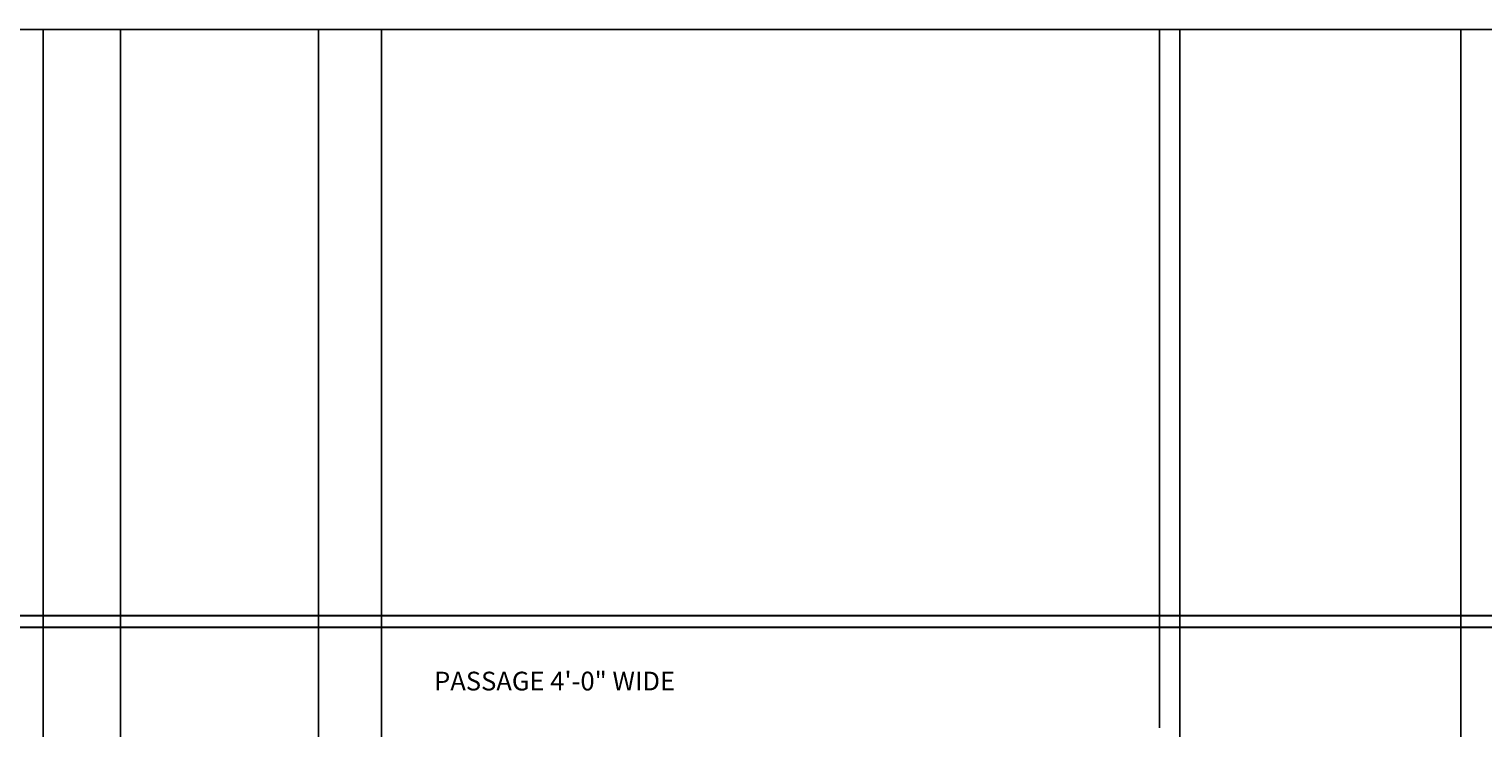
# Model space of a CAD drawing. Units: inches. Extents: x 2330 to 3943, y 1763 to 3461.
# Tile 39 of 40: x 2973 to 3594, y 3163 to 3461. Entities that reach past the tile are written whole.
import ezdxf

# ---------------------------------------------------------------- set-up
doc = ezdxf.new("R2010")
doc.units = ezdxf.units.IN
for name, color, linetype, lineweight in [('A-ANNO-DIMS', 2, 'Continuous', 18), ('A-AREA-IDEN', 7, 'Continuous', 18), ('C-PROP', 7, 'Continuous', 30)]:
    doc.layers.add(name, color=color, linetype=linetype, lineweight=lineweight)
doc.styles.get("Standard").update_dxf_attribs({"font": 'arial.ttf'})
doc.dimstyles.get("Standard").update_dxf_attribs({"dimtxt": 0.18, "dimasz": 0.18, "dimexe": 0.18, "dimexo": 0.0625, "dimgap": 0.09, "dimtad": 0, "dimtih": 1, "dimtoh": 1, "dimdec": 4, "dimzin": 0, "dimdsep": 46, "dimtxsty": 'Standard', "dimcen": 0.09, "dimadec": 0, "dimazin": 0, "dimtfac": 1, "dimtdec": 4, "dimtofl": 0, "dimtmove": 0, "dimatfit": 3, "dimfxl": 1, "dimtolj": 1, "dimtzin": 0, "dimarcsym": 0})

# ---------------------------------------------------------------- blocks, each defined once
blk = doc.blocks.new('*D59')
at = {"layer": 'A-ANNO-DIMS', "color": 0, "lineweight": -2, "transparency": 16777216}
for p, q in [((2415.66, 3210.71), (2415.66, 3461.3)), ((2415.84, 3461.12), (3111.31, 3461.12)), ((3807.48, 3461.12), (3112.01, 3461.12)), ((3807.66, 3210.71), (3807.66, 3461.3))]:
    blk.add_line(p, q, dxfattribs=at)
at = {"layer": 'A-ANNO-DIMS', "color": 0, "transparency": 16777216}
for points in [[(2415.84, 3461.15), (2415.84, 3461.09), (2415.66, 3461.12)], [(3807.48, 3461.15), (3807.48, 3461.09), (3807.66, 3461.12)]]:
    blk.add_solid(points, dxfattribs=at)
at = {"layer": 'Defpoints', "color": 0, "transparency": 16777216}
for p in [(3807.66, 3461.12), (2415.66, 3210.65), (3807.66, 3210.65)]:
    blk.add_point(p, dxfattribs=at)
at = {"layer": 'A-ANNO-DIMS', "color": 0, "transparency": 16777216, "insert": (3111.66, 3461.12), "char_height": 0.18, "attachment_point": 5}
blk.add_mtext('\\A1;1392', dxfattribs=at)
blk = doc.blocks.new('*D61')
at = {"layer": 'A-ANNO-DIMS', "color": 0, "lineweight": -2, "transparency": 16777216}
for p, q in [((2475.66, 3162.71), (2475.66, 3461.3)), ((2475.84, 3461.12), (2965.37, 3461.12)), ((3455.48, 3461.12), (2965.95, 3461.12)), ((3455.66, 3162.71), (3455.66, 3461.3))]:
    blk.add_line(p, q, dxfattribs=at)
at = {"layer": 'A-ANNO-DIMS', "color": 0, "transparency": 16777216}
for points in [[(2475.84, 3461.15), (2475.84, 3461.09), (2475.66, 3461.12)], [(3455.48, 3461.15), (3455.48, 3461.09), (3455.66, 3461.12)]]:
    blk.add_solid(points, dxfattribs=at)
at = {"layer": 'Defpoints', "color": 0, "transparency": 16777216}
for p in [(3455.66, 3461.12), (2475.66, 3162.65), (3455.66, 3162.65)]:
    blk.add_point(p, dxfattribs=at)
at = {"layer": 'A-ANNO-DIMS', "color": 0, "transparency": 16777216, "insert": (2965.66, 3461.12), "char_height": 0.18, "attachment_point": 5}
blk.add_mtext('\\A1;980', dxfattribs=at)
blk = doc.blocks.new('*D69')
at = {"layer": 'A-ANNO-DIMS', "color": 0, "lineweight": -2, "transparency": 16777216}
for p, q in [((3464.39, 2975.89), (3464.39, 3461.3)), ((3464.57, 3461.12), (3524.11, 3461.12)), ((3584.21, 3461.12), (3524.67, 3461.12)), ((3584.39, 2975.89), (3584.39, 3461.3))]:
    blk.add_line(p, q, dxfattribs=at)
at = {"layer": 'A-ANNO-DIMS', "color": 0, "transparency": 16777216}
for points in [[(3464.57, 3461.15), (3464.57, 3461.09), (3464.39, 3461.12)], [(3584.21, 3461.15), (3584.21, 3461.09), (3584.39, 3461.12)]]:
    blk.add_solid(points, dxfattribs=at)
at = {"layer": 'Defpoints', "color": 0, "transparency": 16777216}
for p in [(3584.39, 3461.12), (3464.39, 2975.83), (3584.39, 2975.83)]:
    blk.add_point(p, dxfattribs=at)
at = {"layer": 'A-ANNO-DIMS', "color": 0, "transparency": 16777216, "insert": (3524.39, 3461.12), "char_height": 0.18, "attachment_point": 5}
blk.add_mtext('\\A1;120', dxfattribs=at)
blk = doc.blocks.new('*D87')
at = {"layer": 'A-ANNO-DIMS', "color": 0, "lineweight": -2, "transparency": 16777216}
for p, q in [((2979.12, 3100.1), (2979.12, 3461.3)), ((2979.3, 3461.12), (2995.4, 3461.12)), ((3011.94, 3461.12), (2995.84, 3461.12)), ((3012.12, 3089.6), (3012.12, 3461.3))]:
    blk.add_line(p, q, dxfattribs=at)
at = {"layer": 'A-ANNO-DIMS', "color": 0, "transparency": 16777216}
for points in [[(2979.3, 3461.15), (2979.3, 3461.09), (2979.12, 3461.12)], [(3011.94, 3461.15), (3011.94, 3461.09), (3012.12, 3461.12)]]:
    blk.add_solid(points, dxfattribs=at)
at = {"layer": 'Defpoints', "color": 0, "transparency": 16777216}
for p in [(3012.12, 3461.12), (2979.12, 3100.04), (3012.12, 3089.54)]:
    blk.add_point(p, dxfattribs=at)
at = {"layer": 'A-ANNO-DIMS', "color": 0, "transparency": 16777216, "insert": (2995.62, 3461.12), "char_height": 0.18, "attachment_point": 5}
blk.add_mtext('\\A1;33', dxfattribs=at)
blk = doc.blocks.new('*D94')
at = {"layer": 'A-ANNO-DIMS', "color": 0, "lineweight": -2, "transparency": 16777216}
for p, q in [((3096.66, 3153.71), (3096.66, 3461.3)), ((3096.84, 3461.12), (3109.94, 3461.12)), ((3123.48, 3461.12), (3110.38, 3461.12)), ((3123.66, 3153.71), (3123.66, 3461.3))]:
    blk.add_line(p, q, dxfattribs=at)
at = {"layer": 'A-ANNO-DIMS', "color": 0, "transparency": 16777216}
for points in [[(3096.84, 3461.15), (3096.84, 3461.09), (3096.66, 3461.12)], [(3123.48, 3461.15), (3123.48, 3461.09), (3123.66, 3461.12)]]:
    blk.add_solid(points, dxfattribs=at)
at = {"layer": 'Defpoints', "color": 0, "transparency": 16777216}
for p in [(3123.66, 3461.12), (3096.66, 3153.65), (3123.66, 3153.65)]:
    blk.add_point(p, dxfattribs=at)
at = {"layer": 'A-ANNO-DIMS', "color": 0, "transparency": 16777216, "insert": (3110.16, 3461.12), "char_height": 0.18, "attachment_point": 5}
blk.add_mtext('\\A1;27', dxfattribs=at)

msp = doc.modelspace()

# ---------------------------------------------------------------- linework, layer by layer
at = {"layer": 'C-PROP'}
for p, q in [((2415.6605, 3210.6524), (3807.6605, 3210.6524)), ((2420.6605, 3205.6524), (3802.6605, 3205.6524))]:
    msp.add_line(p, q, dxfattribs=at)

# ---------------------------------------------------------------- texts
at = {"layer": 'A-AREA-IDEN', "insert": (3146.0622, 3186.6856), "char_height": 8, "attachment_point": 1}
msp.add_mtext_dynamic_manual_height_columns('PASSAGE 4\'-0" WIDE', width=157.761408, gutter_width=12.5, heights=[0], dxfattribs=at)

# ---------------------------------------------------------------- dimensions: what is measured, and where the dimension line sits
at = {"layer": 'A-ANNO-DIMS'}
for base, p1, p2, picture, middle in [((3807.6605, 3461.1231), (2415.6605, 3210.6524), (3807.6605, 3210.6524), '*D59', (3111.6605, 3461.1231)), ((3455.6605, 3461.1231), (2475.6605, 3162.6524), (3455.6605, 3162.6524), '*D61', (2965.6605, 3461.1231)), ((3012.1218, 3461.1231), (2979.1218, 3100.0386), (3012.1218, 3089.5386), '*D87', (2995.6218, 3461.1231)), ((3123.6605, 3461.1231), (3096.6605, 3153.6524), (3123.6605, 3153.6524), '*D94', (3110.1605, 3461.1231)), ((3584.3948, 3461.1231), (3464.3948, 2975.8319), (3584.3948, 2975.8319), '*D69', (3524.3948, 3461.1231))]:
    dim = msp.add_linear_dim(base=base, p1=p1, p2=p2, dimstyle='Standard', override={"dimdec": 0, "dimlfac": 1, "dimrnd": 0, "dimzin": 0, "dimdsep": 46, "dimlunit": 2}, dxfattribs=at)
    dim.commit()
    dim.dimension.update_dxf_attribs({"geometry": picture, "text_midpoint": middle})

doc.saveas('drawing.dxf')
